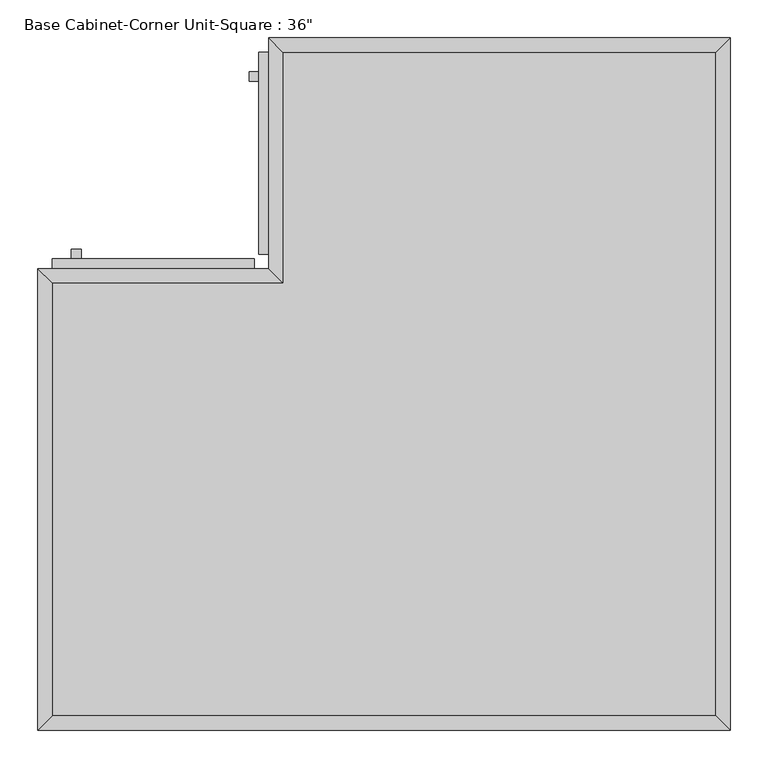
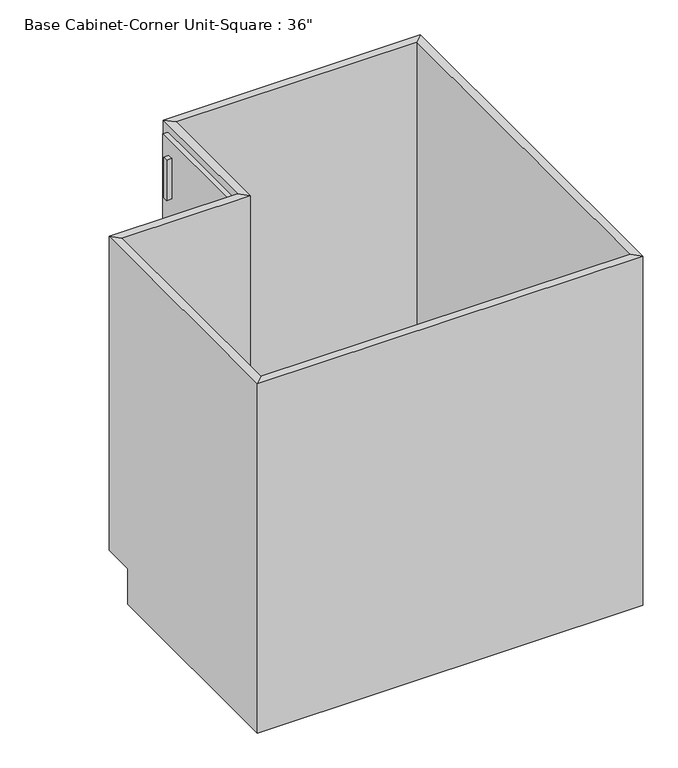
"""IFC4 building model written with IfcOpenShell, lengths in millimetres: furniture geometry."""

from ifc_helpers import new_model, si_unit, frame, origin, place, context, project, spatial, polyline, outline, extrude, faceted_brep, source, transform, mapped, element, save


def furniture_007fecef(model_context):
    return source(origin(), model_context, "Body", "SolidModel", [
        extrude(outline(polyline([(507.6877049, 19.05), (-368.6122951, 19.05), (-368.6122951, 590.55), (-63.8122951, 590.55), (-63.8122951, 895.35), (507.6877049, 895.35), (507.6877049, 19.05)])), frame((0.0, 0.0, 88.9), z_axis=(0.0, 0.0, 1.0), x_axis=(1.0, 0.0, 0.0)), (0.0, 0.0, 1.0), 19.05),
        extrude(outline(polyline([(-101.9122951, 622.3), (-101.9122951, 609.6), (-368.6122951, 609.6), (-368.6122951, 622.3), (-101.9122951, 622.3)])), frame((0.0, 0.0, 107.95), z_axis=(0.0, 0.0, 1.0), x_axis=(1.0, 0.0, 0.0)), (0.0, 0.0, 1.0), 749.3),
        extrude(outline(polyline([(-330.5122951, 635.0), (-330.5122951, 622.3), (-343.2122951, 622.3), (-343.2122951, 635.0), (-330.5122951, 635.0)])), frame((0.0, 0.0, 717.55), z_axis=(0.0, 0.0, 1.0), x_axis=(1.0, 0.0, 0.0)), (0.0, 0.0, 1.0), 101.6),
        extrude(outline(polyline([(-82.8622951, 628.65), (-95.5622951, 628.65), (-95.5622951, 895.35), (-82.8622951, 895.35), (-82.8622951, 628.65)])), frame((0.0, 0.0, 107.95), z_axis=(0.0, 0.0, 1.0), x_axis=(1.0, 0.0, 0.0)), (0.0, 0.0, 1.0), 749.3),
        extrude(outline(polyline([(-95.5622951, 857.25), (-108.2622951, 857.25), (-108.2622951, 869.95), (-95.5622951, 869.95), (-95.5622951, 857.25)])), frame((0.0, 0.0, 717.55), z_axis=(0.0, 0.0, 1.0), x_axis=(1.0, 0.0, 0.0)), (0.0, 0.0, 1.0), 101.6),
        faceted_brep([(-368.6122951, 533.4, 88.9), (-368.6122951, 19.05, 88.9), (507.6877049, 19.05, 88.9), (507.6877049, 895.35, 88.9), (-6.6622951, 895.35, 88.9), (-6.6622951, 533.4, 88.9), (526.7377049, 0.0, 0.0), (-387.6622951, 0.0, 0.0), (-387.6622951, 533.4, 0.0), (-6.6622951, 533.4, 0.0), (-6.6622951, 914.4, 0.0), (526.7377049, 914.4, 0.0), (526.7377049, 0.0, 876.3), (-387.6622951, 0.0, 876.3), (-387.6622951, 609.6, 876.3), (-387.6622951, 609.6, 88.9), (-387.6622951, 533.4, 88.9), (-6.6622951, 914.4, 88.9), (-82.8622951, 914.4, 88.9), (-82.8622951, 914.4, 876.3), (526.7377049, 914.4, 876.3), (507.6877049, 895.35, 876.3), (-63.8122951, 895.35, 876.3), (-63.8122951, 895.35, 88.9), (-63.8122951, 590.55, 876.3), (-63.8122951, 590.55, 88.9), (-82.8622951, 609.6, 876.3), (-82.8622951, 609.6, 88.9), (-368.6122951, 590.55, 876.3), (-368.6122951, 590.55, 88.9), (-368.6122951, 19.05, 876.3), (507.6877049, 19.05, 876.3)], [[[0, 1, 2, 3, 4, 5]], [[6, 7, 8, 9, 10, 11]], [[6, 12, 13, 7]], [[13, 14, 15, 16, 8, 7]], [[8, 16, 0, 5, 9]], [[9, 5, 4, 17, 10]], [[10, 17, 18, 19, 20, 11]], [[20, 12, 6, 11]], [[21, 22, 23, 4, 3]], [[21, 20, 19, 22]], [[18, 17, 4, 23]], [[22, 24, 25, 23]], [[19, 26, 24, 22]], [[18, 27, 26, 19]], [[23, 25, 27, 18]], [[24, 28, 29, 25]], [[26, 14, 28, 24]], [[27, 15, 14, 26]], [[25, 29, 15, 27]], [[28, 30, 1, 0, 29]], [[14, 13, 30, 28]], [[29, 0, 16, 15]], [[30, 31, 2, 1]], [[13, 12, 31, 30]], [[3, 2, 31, 21]], [[21, 31, 12, 20]]]),
    ])


if __name__ == "__main__":
    model = new_model("IFC4")
    model_context = context("Model", 3, world=origin())
    ifc_project = project(units=[si_unit("LENGTHUNIT", "METRE", prefix="MILLI")], contexts=[model_context])
    site = spatial("IfcSite", under=ifc_project)
    building = spatial("IfcBuilding", under=site)
    placement = place(None, origin())
    furniture_shape = furniture_007fecef(model_context)
    element("IfcFurniture", 1, ObjectType="Base Cabinet-Corner Unit-Square : 36\"", at=placement, inside=building, context=model_context, shape_type="MappedRepresentation", body=[
        mapped(furniture_shape, transform((0.0, 0.0, 0.0), x_axis=(1.0, 0.0, 0.0), y_axis=(0.0, 1.0, 0.0), z_axis=(0.0, 0.0, 1.0))),
    ])
    save(model, "model.ifc")

# Revit data of these elements
# Type "Base Cabinet-Corner Unit-Square : 36\""
#   Assembly Code = "C1030410"
#   Depth = 2' - 0"
#   Height = 2' - 10 1/2"
#   Toe Depth = 0' - 3"
#   Toe Height = 0' - 3 1/2"
#   Width = 3' - 0"
#   Cabinet Material = Cabinets
#   Door/Drawer Material = Cabinets
#   Handle Material = Cabinets - Handles
#   Default Elevation = 0
# Element 1 (IfcFurniture, "Base Cabinet-Corner Unit-Square : 36\"")
#   Materials on its faces: "Cabinets", "Cabinets - Handles"
# Materials
#   "Cabinets": colour RGB 249 249 249, transparency 0
#   "Cabinets - Handles": colour RGB 57 57 57, transparency 0
